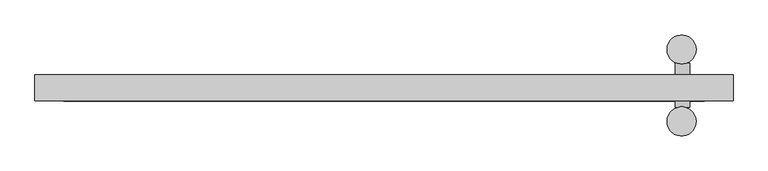
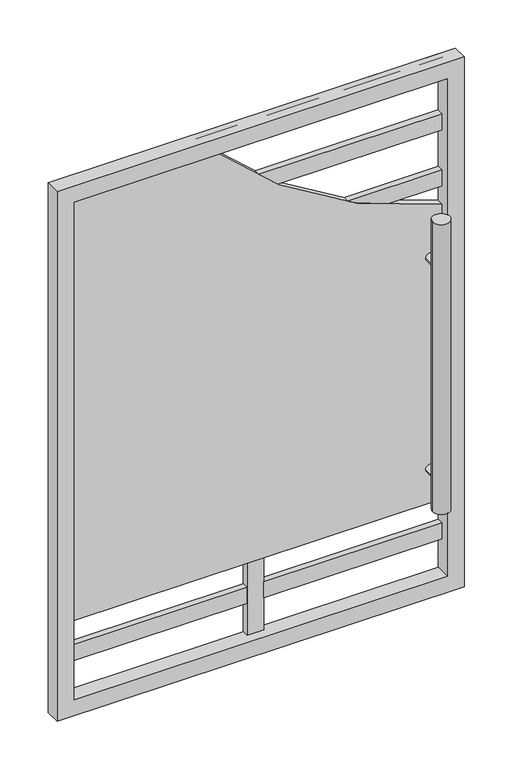
"""IFC4 building model written with IfcOpenShell, lengths in millimetres: proxy geometry."""

from ifc_helpers import new_model, si_unit, point, frame, frame_2d, origin, place, context, project, spatial, polyline, circle_curve, trimmed, segment, composite_curve, outline, extrude, source, transform, mapped, element, save


def generic_models_918bcdec(model_context):
    return source(origin(), model_context, "Body", "SweptSolid", [
        extrude(outline(polyline([(0.0, -1219.2), (0.0, 0.0), (1676.4, 0.0), (1676.4, -1219.2), (0.0, -1219.2)]), holes=[polyline([(50.8, -1168.4), (1625.6, -1168.4), (1625.6, -50.8), (50.8, -50.8), (50.8, -1168.4)])]), frame((0.0, -46.0617726, 0.0), z_axis=(0.0, 1.0, 0.0), x_axis=(0.0, 0.0, 1.0)), (0.0, 0.0, 1.0), 46.0617726),
        extrude(outline(composite_curve([segment(polyline([(1625.6, -1168.4), (279.4, -1168.4), (279.4, -50.8), (1212.1744192, -50.8)]), True, "CONTINUOUS"), segment(trimmed(circle_curve(frame_2d((2582.6324877, 299.8877691)), 1414.6155764), [point((1212.1744192, -50.8))], [point((1625.6, -741.8540639))], True, "CARTESIAN"), True, "CONTINUOUS"), segment(polyline([(1625.6, -741.8540639), (1625.6, -1168.4)]), True, "CONTINUOUS")], self_intersect=False)), frame((0.0, -19.05, 0.0), z_axis=(0.0, 1.0, 0.0), x_axis=(0.0, 0.0, 1.0)), (0.0, 0.0, 1.0), 19.05),
        extrude(outline(composite_curve([segment(polyline([(1676.4, -50.8), (1676.4, -786.3350015)]), True, "CONTINUOUS"), segment(trimmed(circle_curve(frame_2d((2582.6324877, 299.8877691)), 1414.6155764), [point((1676.4, -786.3350015))], [point((1625.6, -741.8540639))], False, "CARTESIAN"), True, "CONTINUOUS"), segment(polyline([(1625.6, -741.8540639), (1625.6, -50.8), (1676.4, -50.8)]), True, "CONTINUOUS")], self_intersect=False)), frame((0.0, -19.05, 0.0), z_axis=(0.0, 1.0, 0.0), x_axis=(0.0, 0.0, 1.0)), (0.0, 0.0, 1.0), 19.05),
        extrude(outline(composite_curve([segment(polyline([(1498.6, -50.8), (1498.6, -608.963591)]), True, "CONTINUOUS"), segment(trimmed(circle_curve(frame_2d((2582.6324877, 299.8877691)), 1414.6155764), [point((1498.6, -608.963591))], [point((1447.8, -544.6786605))], False, "CARTESIAN"), True, "CONTINUOUS"), segment(polyline([(1447.8, -544.6786605), (1447.8, -50.8), (1498.6, -50.8)]), True, "CONTINUOUS")], self_intersect=False)), frame((0.0, -19.05, 0.0), z_axis=(0.0, 1.0, 0.0), x_axis=(0.0, 0.0, 1.0)), (0.0, 0.0, 1.0), 19.05),
        extrude(outline(composite_curve([segment(polyline([(1320.8, -50.8), (1320.8, -339.5776342)]), True, "CONTINUOUS"), segment(trimmed(circle_curve(frame_2d((2582.6324877, 299.8877691)), 1414.6155764), [point((1320.8, -339.5776342))], [point((1270.0, -227.4955652))], False, "CARTESIAN"), True, "CONTINUOUS"), segment(polyline([(1270.0, -227.4955652), (1270.0, -50.8), (1320.8, -50.8)]), True, "CONTINUOUS")], self_intersect=False)), frame((0.0, -19.05, 0.0), z_axis=(0.0, 1.0, 0.0), x_axis=(0.0, 0.0, 1.0)), (0.0, 0.0, 1.0), 19.05),
        extrude(outline(polyline([(-635.0, -19.05), (-1168.4, -19.05), (-1168.4, 0.0), (-635.0, 0.0), (-635.0, -19.05)])), frame((0.0, 0.0, 152.4), z_axis=(0.0, 0.0, 1.0), x_axis=(1.0, 0.0, 0.0)), (0.0, 0.0, 1.0), 50.8),
        extrude(outline(polyline([(-50.8, -19.05), (-584.2, -19.05), (-584.2, 0.0), (-50.8, 0.0), (-50.8, -19.05)])), frame((0.0, 0.0, 152.4), z_axis=(0.0, 0.0, 1.0), x_axis=(1.0, 0.0, 0.0)), (0.0, 0.0, 1.0), 50.8),
        extrude(outline(polyline([(-584.2, -19.05), (-635.0, -19.05), (-635.0, 0.0), (-584.2, 0.0), (-584.2, -19.05)])), frame((0.0, 0.0, 50.8), z_axis=(0.0, 0.0, 1.0), x_axis=(1.0, 0.0, 0.0)), (0.0, 0.0, 1.0), 228.6),
        extrude(outline(composite_curve([segment(trimmed(circle_curve(frame_2d((-89.7949058, 43.7785099)), 25.4), [point((-64.3949058, 43.7785099))], [point((-115.1949058, 43.7785099))], False, "CARTESIAN"), True, "CONTINUOUS"), segment(trimmed(circle_curve(frame_2d((-89.7949058, 43.7785099)), 25.4), [point((-115.1949058, 43.7785099))], [point((-64.3949058, 43.7785099))], False, "CARTESIAN"), True, "CONTINUOUS")], self_intersect=False)), frame((0.0, 0.0, 279.4), z_axis=(0.0, 0.0, 1.0), x_axis=(1.0, 0.0, 0.0)), (0.0, 0.0, 1.0), 889.0),
        extrude(outline(composite_curve([segment(trimmed(circle_curve(frame_2d((-89.7949058, -81.8785099)), 25.4), [point((-64.3949058, -81.8785099))], [point((-115.1949058, -81.8785099))], False, "CARTESIAN"), True, "CONTINUOUS"), segment(trimmed(circle_curve(frame_2d((-89.7949058, -81.8785099)), 25.4), [point((-115.1949058, -81.8785099))], [point((-64.3949058, -81.8785099))], False, "CARTESIAN"), True, "CONTINUOUS")], self_intersect=False)), frame((0.0, 0.0, 298.8472671), z_axis=(0.0, 0.0, 1.0), x_axis=(1.0, 0.0, 0.0)), (0.0, 0.0, 1.0), 917.3073645),
        extrude(outline(composite_curve([segment(trimmed(circle_curve(frame_2d((1058.3458504, -88.119132)), 12.7), [point((1058.3458504, -75.419132))], [point((1058.3458504, -100.819132))], False, "CARTESIAN"), True, "CONTINUOUS"), segment(trimmed(circle_curve(frame_2d((1058.3458504, -88.119132)), 12.7), [point((1058.3458504, -100.819132))], [point((1058.3458504, -75.419132))], False, "CARTESIAN"), True, "CONTINUOUS")], self_intersect=False)), frame((0.0, -57.15, 0.0), z_axis=(0.0, 1.0, 0.0), x_axis=(0.0, 0.0, 1.0)), (0.0, 0.0, 1.0), 76.6172039),
        extrude(outline(composite_curve([segment(trimmed(circle_curve(frame_2d((389.4541496, -88.119132)), 12.7), [point((389.4541496, -75.419132))], [point((389.4541496, -100.819132))], False, "CARTESIAN"), True, "CONTINUOUS"), segment(trimmed(circle_curve(frame_2d((389.4541496, -88.119132)), 12.7), [point((389.4541496, -100.819132))], [point((389.4541496, -75.419132))], False, "CARTESIAN"), True, "CONTINUOUS")], self_intersect=False)), frame((0.0, -57.15, 0.0), z_axis=(0.0, 1.0, 0.0), x_axis=(0.0, 0.0, 1.0)), (0.0, 0.0, 1.0), 76.7981605),
    ])


if __name__ == "__main__":
    model = new_model("IFC4")
    model_context = context("Model", 3, world=origin())
    ifc_project = project(units=[si_unit("LENGTHUNIT", "METRE", prefix="MILLI")], contexts=[model_context])
    site = spatial("IfcSite", under=ifc_project)
    building = spatial("IfcBuilding", under=site)
    placement = place(None, origin())
    generic_models_shape = generic_models_918bcdec(model_context)
    element("IfcBuildingElementProxy", 1, Name="Generic Models", at=placement, inside=building, context=model_context, shape_type="MappedRepresentation", body=[
        mapped(generic_models_shape, transform((0.0, 0.0, 0.0), x_axis=(1.0, 0.0, 0.0), y_axis=(0.0, 1.0, 0.0), z_axis=(0.0, 0.0, 1.0))),
    ])
    save(model, "model.ifc")

# Revit data of these elements
# Type
#   sheet = Door - Panel
#   pipe = Door - Panel
#   handal = Door - Panel
#   faram = Door - Panel
#   Default Elevation = 0
# Element 1 (IfcBuildingElementProxy)
#   Materials on its faces: "Earth", "Door - Panel"
# Materials
#   "Door - Panel": class "Wood", colour RGB 210 159 95, transparency 0, Cost = 0
#   "Earth": class "Generic", colour RGB 97 75 62, transparency 0, Description = "Soil", Cost = 0
